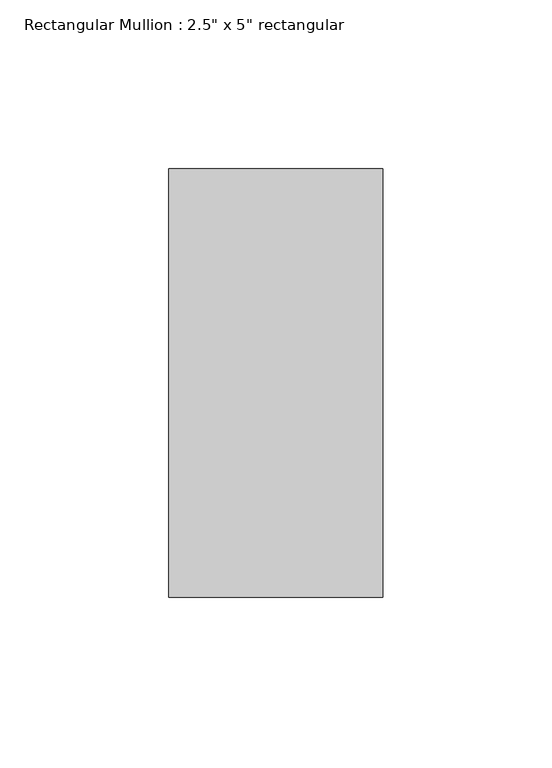
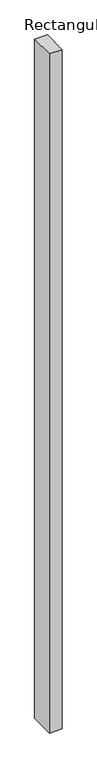
"""IFC4 building model written with IfcOpenShell, lengths in millimetres: member geometry."""

from ifc_helpers import new_model, si_unit, frame, origin, place, context, project, spatial, polyline, outline, extrude, source, transform, mapped, element, save


def member_2b402daf(model_context):
    return source(origin(), model_context, "Body", "SweptSolid", [
        extrude(outline(polyline([(0.0, 63.5), (0.0, -63.5), (-63.5, -63.5), (-63.5, 63.5), (0.0, 63.5)])), frame((0.0, 0.0, -3562.35), z_axis=(0.0, 0.0, 1.0), x_axis=(1.0, 0.0, 0.0)), (0.0, 0.0, 1.0), 3562.35),
    ])


if __name__ == "__main__":
    model = new_model("IFC4")
    model_context = context("Model", 3, world=origin())
    ifc_project = project(units=[si_unit("LENGTHUNIT", "METRE", prefix="MILLI")], contexts=[model_context])
    site = spatial("IfcSite", under=ifc_project)
    building = spatial("IfcBuilding", under=site)
    placement = place(None, origin())
    member_shape = member_2b402daf(model_context)
    element("IfcMember", 1, ObjectType="Rectangular Mullion : 2.5\" x 5\" rectangular", at=placement, inside=building, context=model_context, shape_type="MappedRepresentation", body=[
        mapped(member_shape, transform((0.0, 0.0, 0.0), x_axis=(1.0, 0.0, 0.0), y_axis=(0.0, 1.0, 0.0), z_axis=(0.0, 0.0, 1.0))),
    ])
    save(model, "model.ifc")

# Revit data of these elements
# Type "Rectangular Mullion : 2.5\" x 5\" rectangular"
#   built-in parameter 1007304 = 0.416667 (stored number, unit not read)
#   built-in parameter 1007301 = 0.104167 (stored number, unit not read)
#   built-in parameter 1007300 = 0.104167 (stored number, unit not read)
# Element 1 (IfcMember, "Rectangular Mullion : 2.5\" x 5\" rectangular")
#   Materials on its faces: "Aluminum"
# Materials
#   "Aluminum": class "Metal", colour RGB 247 247 247, transparency 0, Description = "Aluminum 6061", Cost = 0
